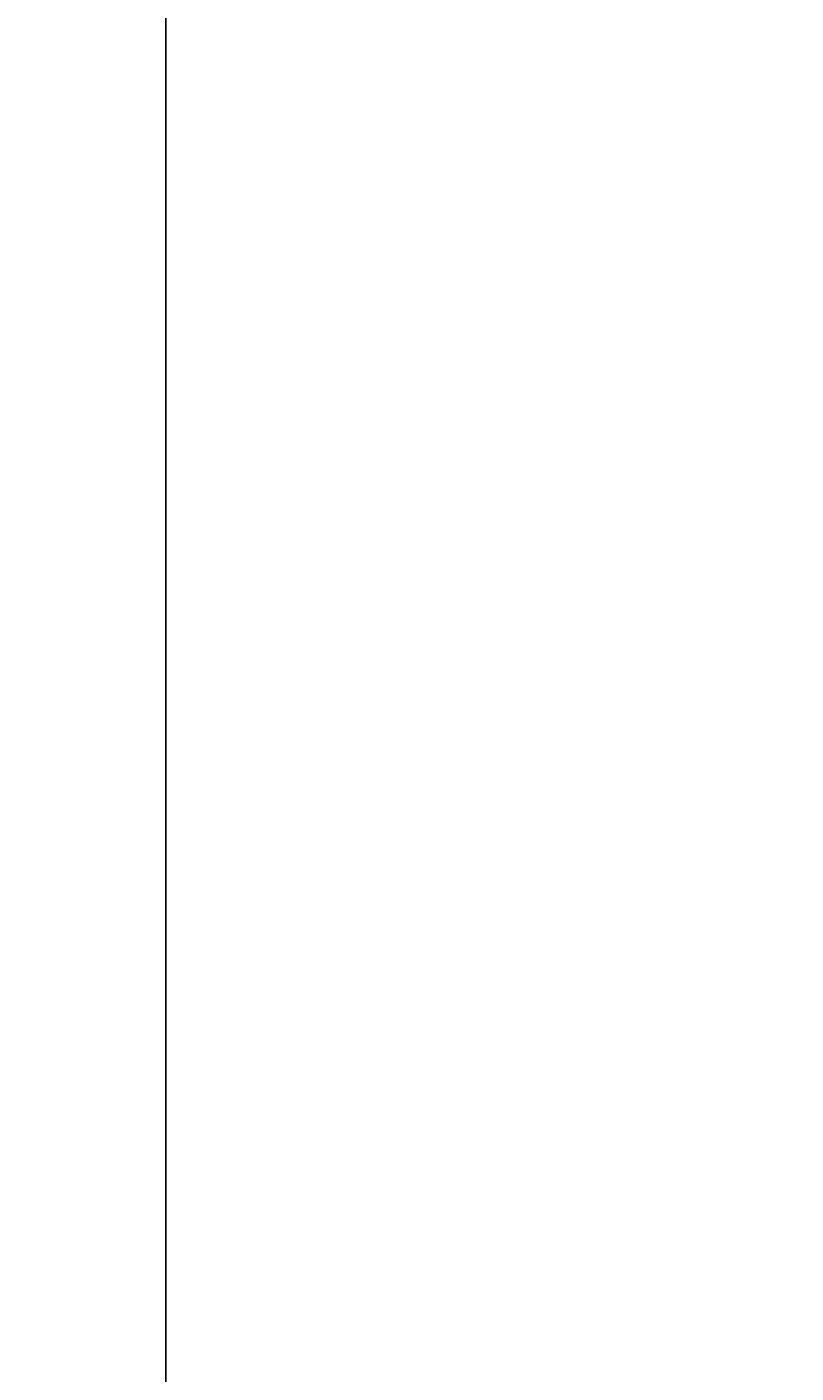
# Model space of a CAD drawing. Units: inches. Extents: x 1441 to 2460, y 1648 to 2683.
# Tile 24 of 35: x 1792 to 1810, y 2253 to 2284. Entities that reach past the tile are written whole.
import ezdxf

# ---------------------------------------------------------------- set-up
doc = ezdxf.new("R2010")
doc.units = ezdxf.units.IN
doc.layers.add('A-ANNO-DIMS', color=2, linetype='Continuous', lineweight=18)
doc.styles.get("Standard").update_dxf_attribs({"font": 'arial.ttf'})
doc.dimstyles.get("Standard").update_dxf_attribs({"dimtxt": 0.18, "dimasz": 0.18, "dimexe": 0.18, "dimexo": 0.0625, "dimgap": 0.09, "dimtad": 0, "dimtih": 1, "dimtoh": 1, "dimdec": 4, "dimzin": 0, "dimdsep": 46, "dimtxsty": 'Standard', "dimcen": 0.09, "dimadec": 0, "dimazin": 0, "dimtfac": 1, "dimtdec": 4, "dimtofl": 0, "dimtmove": 0, "dimatfit": 3, "dimfxl": 1, "dimtolj": 1, "dimtzin": 0, "dimarcsym": 0})

# ---------------------------------------------------------------- blocks, each defined once
blk = doc.blocks.new('*D22')
at = {"layer": 'A-ANNO-DIMS', "color": 0, "lineweight": -2, "transparency": 16777216}
for p, q in [((1809.14, 2287.87), (1795.269, 2287.87)), ((1795.449, 2287.69), (1795.449, 2242.209)), ((1795.449, 2196.362), (1795.449, 2241.843)), ((1809.14, 2196.182), (1795.269, 2196.182))]:
    blk.add_line(p, q, dxfattribs=at)
at = {"layer": 'A-ANNO-DIMS', "color": 0, "transparency": 16777216}
for points in [[(1795.419, 2287.69), (1795.479, 2287.69), (1795.449, 2287.87)], [(1795.419, 2196.362), (1795.479, 2196.362), (1795.449, 2196.182)]]:
    blk.add_solid(points, dxfattribs=at)
at = {"layer": 'Defpoints', "color": 0, "transparency": 16777216}
for p in [(1795.449, 2287.87), (1809.202, 2287.87), (1809.202, 2196.182)]:
    blk.add_point(p, dxfattribs=at)
at = {"layer": 'A-ANNO-DIMS', "color": 0, "transparency": 16777216, "insert": (1795.449, 2242.026), "char_height": 0.18, "attachment_point": 5}
blk.add_mtext('\\A1;DOUBLE BED 92 TYP.', dxfattribs=at)
blk = doc.blocks.new('*D67')
at = {"layer": 'A-ANNO-DIMS', "color": 0, "lineweight": -2, "transparency": 16777216}
for p, q in [((1889.448, 2298.695), (1916.216, 2298.695)), ((1916.036, 2298.515), (1916.036, 2055.938)), ((1916.036, 1812.997), (1916.036, 2055.574)), ((1758.224, 1812.817), (1916.216, 1812.817))]:
    blk.add_line(p, q, dxfattribs=at)
at = {"layer": 'A-ANNO-DIMS', "color": 0, "transparency": 16777216}
for points in [[(1916.006, 2298.515), (1916.066, 2298.515), (1916.036, 2298.695)], [(1916.006, 1812.997), (1916.066, 1812.997), (1916.036, 1812.817)]]:
    blk.add_solid(points, dxfattribs=at)
at = {"layer": 'Defpoints', "color": 0, "transparency": 16777216}
for p in [(1889.386, 2298.695), (1916.036, 2298.695), (1758.161, 1812.817)]:
    blk.add_point(p, dxfattribs=at)
at = {"layer": 'A-ANNO-DIMS', "color": 0, "transparency": 16777216, "insert": (1916.036, 2055.756), "char_height": 0.18, "attachment_point": 5}
blk.add_mtext('\\A1;485.9', dxfattribs=at)

msp = doc.modelspace()

# ---------------------------------------------------------------- dimensions: what is measured, and where the dimension line sits
at = {"layer": 'A-ANNO-DIMS'}
dim = msp.add_linear_dim(base=(1916.0359, 2298.6952), p1=(1758.1615, 1812.8171), p2=(1889.3859, 2298.6952), angle=90, dimstyle='Standard', override={"dimdec": 1, "dimlfac": 1, "dimrnd": 0, "dimzin": 0, "dimdsep": 46, "dimlunit": 2}, dxfattribs=at)
dim.commit()
dim.dimension.update_dxf_attribs({"geometry": '*D67', "text_midpoint": (1916.0359, 2055.7561)})
dim = msp.add_linear_dim(base=(1795.4489, 2287.8701), p1=(1809.2021, 2196.1822), p2=(1809.2021, 2287.8701), angle=90, text='DOUBLE BED <> TYP.', dimstyle='Standard', override={"dimdec": 0, "dimlfac": 1, "dimrnd": 0, "dimzin": 0, "dimdsep": 46, "dimlunit": 2}, dxfattribs=at)
dim.commit()
dim.dimension.update_dxf_attribs({"geometry": '*D22', "text_midpoint": (1795.4489, 2242.0262)})

doc.saveas('drawing.dxf')
